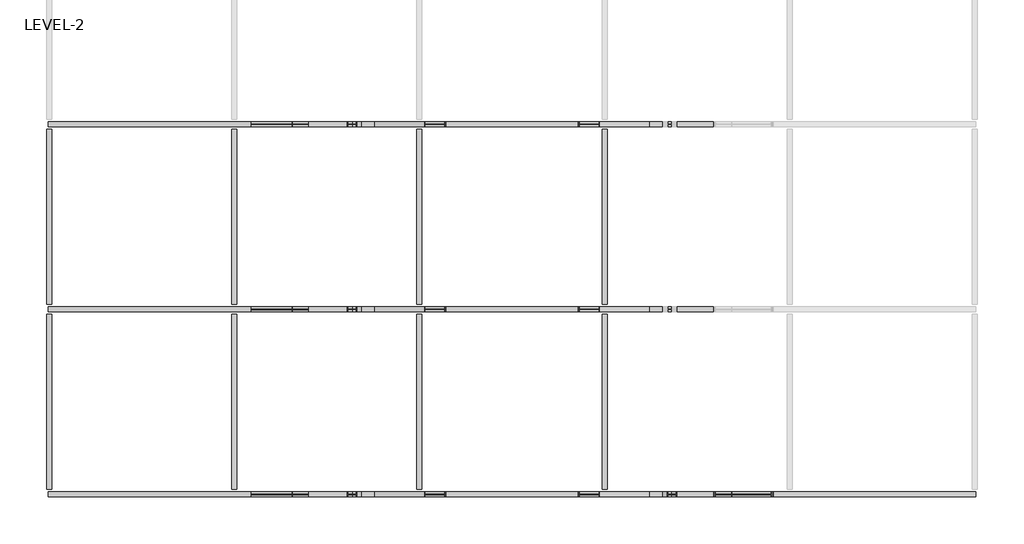
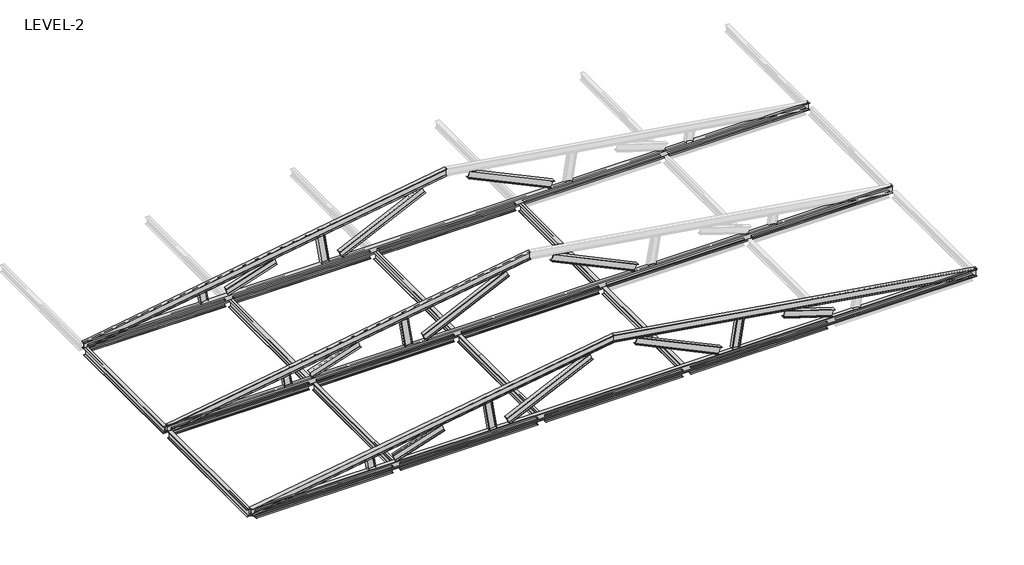
# One storey, part 1 of 3: 42 beams.
"""IFC4 building model written with IfcOpenShell, lengths in millimetres."""

from ifc_helpers import new_model, si_unit, frame, origin, place, context, project, spatial, polyline, circle_curve, ellipse_curve, transform, mapped, element, save
from ifc_brep_helpers import plane_surface, revolved_surface, advanced_brep
from components import ub_universal_beams_ub305x165x40_616d6e4e, ub_universal_beams_ub305x165x40_3f70edd5, ub_universal_beams_ub305x165x40_c9eec61f, ub_universal_beams_ub305x165x40_c956ba20, ub_universal_beams_ub305x165x40_f58164a9, ub_universal_beams_ub305x165x40_ef0a91e2, ub_universal_beams_ub305x165x40_83ed4f69, ub_universal_beams_ub305x165x40_46a3dc55, ub_universal_beams_ub305x165x40_0b6a72e4, ub_universal_beams_ub305x165x40_05d28e63

model = new_model("IFC4")

# Units and contexts
model_context = context("Model", 3, world=origin())
ifc_project = project(units=[si_unit("LENGTHUNIT", "METRE", prefix="MILLI")], contexts=[model_context])

# Site, building, storey
site = spatial("IfcSite", under=ifc_project)
building = spatial("IfcBuilding", under=site)
storey = spatial("IfcBuildingStorey", under=building, Name="LEVEL-2", Elevation=4267.0)

# Beams
placement = place(None, origin())
element("IfcBeam", 1, ObjectType="UB-Universal Beams : UB305x165x40", at=placement, inside=storey, context=model_context, shape_type="AdvancedBrep", body=[
    advanced_brep(
    [(-18518.3117021, -14245.9765895, 4127.2241081), (-18516.724958, -14245.9765895, 4117.1482834), (-18516.724958, -14410.9765895, 4117.1482834), (-18518.3117021, -14410.9765895, 4127.2241081), (-18518.3117021, -14340.3765895, 4127.2241081), (-18519.696214, -14331.4765895, 4136.0157591), (-18560.9515593, -14331.4765895, 4397.9872012), (-18562.3360712, -14340.3765895, 4406.7788522), (-18562.3360712, -14410.9765895, 4406.7788522), (-18563.9228153, -14410.9765895, 4416.8546768), (-18563.9228153, -14245.9765895, 4416.8546768), (-18562.3360712, -14245.9765895, 4406.7788522), (-18562.3360712, -14316.5765895, 4406.7788522), (-18560.9515593, -14325.4765895, 4397.9872012), (-18519.696214, -14325.4765895, 4136.0157591), (-18518.3117021, -14316.5765895, 4127.2241081), (-3300.3332854, -14316.5765895, 6523.7561422), (-3300.3332854, -14245.9765895, 6523.7561422), (-3300.3332854, -14325.4765895, 6532.7658266), (-3300.3332854, -14325.4765895, 6801.2341734), (-3300.3332854, -14316.5765895, 6810.2438578), (-3300.3332854, -14245.9765895, 6810.2438578), (-3300.3332854, -14245.9765895, 6820.5695634), (-3300.3332854, -14410.9765895, 6820.5695634), (-3300.3332854, -14410.9765895, 6810.2438578), (-3300.3332854, -14340.3765895, 6810.2438578), (-3300.3332854, -14331.4765895, 6801.2341734), (-3300.3332854, -14331.4765895, 6532.7658266), (-3300.3332854, -14340.3765895, 6523.7561422), (-3300.3332854, -14410.9765895, 6523.7561422), (-3300.3332854, -14410.9765895, 6513.4304366), (-3300.3332854, -14245.9765895, 6513.4304366)],
    [
        (0, 1),
        (1, 2),
        (2, 3),
        (3, 4),
        (4, 5, circle_curve(frame((-18519.696214, -14340.3765895, 4136.0157591), z_axis=(0.9878259507117182, 0.0, 0.1555631418443652), x_axis=(0.0, -1.0, 0.0)), 8.9)),
        (5, 6),
        (6, 7, circle_curve(frame((-18560.9515593, -14340.3765895, 4397.9872012), z_axis=(0.9878259507117182, 0.0, 0.1555631418443652), x_axis=(0.0, -1.0, 0.0)), 8.9)),
        (7, 8),
        (8, 9),
        (9, 10),
        (10, 11),
        (11, 12),
        (12, 13, circle_curve(frame((-18560.9515593, -14316.5765895, 4397.9872012), z_axis=(0.9878259507117182, 0.0, 0.1555631418443652), x_axis=(0.0, -1.0, 0.0)), 8.9)),
        (13, 14),
        (14, 15, circle_curve(frame((-18519.696214, -14316.5765895, 4136.0157591), z_axis=(0.9878259507117182, 0.0, 0.1555631418443652), x_axis=(0.0, -1.0, 0.0)), 8.9)),
        (15, 0),
        (16, 17),
        (17, 0),
        (15, 16),
        (18, 16, ellipse_curve(frame((-3300.3332854, -14316.5765895, 6532.7658266), z_axis=(1.0, 0.0, 0.0), x_axis=(0.0, 0.0, -1.0)), 9.0096843, 8.9)),
        (14, 18),
        (19, 18),
        (13, 19),
        (20, 19, ellipse_curve(frame((-3300.3332854, -14316.5765895, 6801.2341734), z_axis=(1.0, 0.0, 0.0), x_axis=(0.0, 0.0, -1.0)), 9.0096843, 8.9)),
        (12, 20),
        (21, 20),
        (11, 21),
        (22, 21),
        (10, 22),
        (23, 22),
        (9, 23),
        (24, 23),
        (8, 24),
        (25, 24),
        (7, 25),
        (26, 25, ellipse_curve(frame((-3300.3332854, -14340.3765895, 6801.2341734), z_axis=(1.0, 0.0, 0.0), x_axis=(0.0, 0.0, -1.0)), 9.0096843, 8.9)),
        (6, 26),
        (27, 26),
        (5, 27),
        (28, 27, ellipse_curve(frame((-3300.3332854, -14340.3765895, 6532.7658266), z_axis=(1.0, 0.0, 0.0), x_axis=(0.0, 0.0, -1.0)), 9.0096843, 8.9)),
        (4, 28),
        (29, 28),
        (3, 29),
        (30, 29),
        (2, 30),
        (31, 30),
        (1, 31),
        (17, 31),
    ],
    [
        plane_surface(frame((-18540.3238866, -14328.4765895, 4267.0014801), z_axis=(-0.9878259507117182, 0.0, -0.1555631418443652), x_axis=(-0.1555631418443652, 0.0, 0.9878259507117182))),
        plane_surface(frame((-3278.3304997, -14245.9765895, 6527.2211478), z_axis=(-0.1555631418443652, 0.0, 0.9878259507117182), x_axis=(-0.9878259507117182, 0.0, -0.1555631418443652))),
        revolved_surface(polyline([(-18519.696214059466, -14325.4765895, 4136.015759042602), (-3298.948773435937, -14325.4765895, 6532.983859928199)]), (-3279.7150116, -14316.5765895, 6536.0127988), (-0.9878259507117182, 0.0, -0.1555631418443652)),
        plane_surface(frame((-3279.7150116, -14325.4765895, 6536.0127988), z_axis=(0.0, 1.0, 0.0), x_axis=(-0.9878259507117182, 0.0, -0.1555631418443652))),
        revolved_surface(polyline([(-18560.95155929262, -14325.4765895, 4397.98720115313), (-3298.948773431581, -14325.4765895, 6801.452206800539)]), (-3320.9703569, -14316.5765895, 6797.9842409), (-0.9878259507117182, 0.0, -0.1555631418443652)),
        plane_surface(frame((-3322.3548688, -14316.5765895, 6806.7758919), z_axis=(0.1555631418443652, 0.0, -0.9878259507117182), x_axis=(-0.9878259507117182, 0.0, -0.1555631418443652))),
        plane_surface(frame((-3322.3548688, -14245.9765895, 6806.7758919), z_axis=(0.0, 1.0, 0.0), x_axis=(-0.9878259507117182, 0.0, -0.1555631418443652))),
        plane_surface(frame((-3323.9416129, -14245.9765895, 6816.8517166), z_axis=(-0.1555631418443652, 0.0, 0.9878259507117182), x_axis=(-0.9878259507117182, 0.0, -0.1555631418443652))),
        plane_surface(frame((-3323.9416129, -14410.9765895, 6816.8517166), z_axis=(0.0, -1.0, 0.0), x_axis=(-0.9878259507117182, 0.0, -0.1555631418443652))),
        plane_surface(frame((-3322.3548688, -14410.9765895, 6806.7758919), z_axis=(0.1555631418443652, 0.0, -0.9878259507117182), x_axis=(-0.9878259507117182, 0.0, -0.1555631418443652))),
        revolved_surface(polyline([(-18560.95155929262, -14349.2765895, 4397.98720115313), (-3298.948773431581, -14349.2765895, 6801.452206800539)]), (-3320.9703569, -14340.3765895, 6797.9842409), (-0.9878259507117182, 0.0, -0.1555631418443652)),
        plane_surface(frame((-3320.9703569, -14331.4765895, 6797.9842409), z_axis=(0.0, -1.0, 0.0), x_axis=(-0.9878259507117182, 0.0, -0.1555631418443652))),
        revolved_surface(polyline([(-18519.696214059466, -14349.2765895, 4136.015759042602), (-3298.948773435937, -14349.2765895, 6532.983859928199)]), (-3279.7150116, -14340.3765895, 6536.0127988), (-0.9878259507117182, 0.0, -0.1555631418443652)),
        plane_surface(frame((-3278.3304997, -14340.3765895, 6527.2211478), z_axis=(-0.1555631418443652, 0.0, 0.9878259507117182), x_axis=(-0.9878259507117182, 0.0, -0.1555631418443652))),
        plane_surface(frame((-3278.3304997, -14410.9765895, 6527.2211478), z_axis=(0.0, -1.0, 0.0), x_axis=(-0.9878259507117182, 0.0, -0.1555631418443652))),
        plane_surface(frame((-3276.7437556, -14410.9765895, 6517.1453232), z_axis=(0.1555631418443652, 0.0, -0.9878259507117182), x_axis=(-0.9878259507117182, 0.0, -0.1555631418443652))),
        plane_surface(frame((-3276.7437556, -14245.9765895, 6517.1453232), z_axis=(0.0, 1.0, 0.0), x_axis=(-0.9878259507117182, 0.0, -0.1555631418443652))),
        plane_surface(frame((-3300.3332854, -14328.4765895, 6820.5695634), z_axis=(1.0, 0.0, 0.0), x_axis=(0.0, -1.0, 0.0))),
    ],
    [
        (0, [[1, 2, 3, 4, 5, 6, 7, 8, 9, 10, 11, 12, 13, 14, 15, 16]]),
        (1, [[17, 18, -16, 19]]),
        (2, [[20, -19, -15, 21]]),
        (3, [[22, -21, -14, 23]]),
        (4, [[24, -23, -13, 25]]),
        (5, [[26, -25, -12, 27]]),
        (6, [[28, -27, -11, 29]]),
        (7, [[30, -29, -10, 31]]),
        (8, [[32, -31, -9, 33]]),
        (9, [[34, -33, -8, 35]]),
        (10, [[36, -35, -7, 37]]),
        (11, [[38, -37, -6, 39]]),
        (12, [[40, -39, -5, 41]]),
        (13, [[42, -41, -4, 43]]),
        (14, [[44, -43, -3, 45]]),
        (15, [[46, -45, -2, 47]]),
        (16, [[48, -47, -1, -18]]),
        (17, [[-17, -20, -22, -24, -26, -28, -30, -32, -34, -36, -38, -40, -42, -44, -46, -48]]),
    ],
),
])
element("IfcBeam", 2, ObjectType="UB-Universal Beams : UB305x165x40", at=placement, inside=storey, context=model_context, shape_type="AdvancedBrep", body=[
    advanced_brep(
    [(11917.6451312, -14245.9765895, 4127.2241081), (11917.6451312, -14316.5765895, 4127.2241081), (11919.0296431, -14325.4765895, 4136.0157591), (11960.2849884, -14325.4765895, 4397.9872012), (11961.6695003, -14316.5765895, 4406.7788522), (11961.6695003, -14245.9765895, 4406.7788522), (11963.2562444, -14245.9765895, 4416.8546768), (11963.2562444, -14410.9765895, 4416.8546768), (11961.6695003, -14410.9765895, 4406.7788522), (11961.6695003, -14340.3765895, 4406.7788522), (11960.2849884, -14331.4765895, 4397.9872012), (11919.0296431, -14331.4765895, 4136.0157591), (11917.6451312, -14340.3765895, 4127.2241081), (11917.6451312, -14410.9765895, 4127.2241081), (11916.0583871, -14410.9765895, 4117.1482834), (11916.0583871, -14245.9765895, 4117.1482834), (-3300.3332854, -14245.9765895, 6523.7561422), (-3300.3332854, -14316.5765895, 6523.7561422), (-3300.3332854, -14325.4765895, 6532.7658266), (-3300.3332854, -14325.4765895, 6801.2341734), (-3300.3332854, -14316.5765895, 6810.2438578), (-3300.3332854, -14245.9765895, 6810.2438578), (-3300.3332854, -14245.9765895, 6820.5695634), (-3300.3332854, -14410.9765895, 6820.5695634), (-3300.3332854, -14410.9765895, 6810.2438578), (-3300.3332854, -14340.3765895, 6810.2438578), (-3300.3332854, -14331.4765895, 6801.2341734), (-3300.3332854, -14331.4765895, 6532.7658266), (-3300.3332854, -14340.3765895, 6523.7561422), (-3300.3332854, -14410.9765895, 6523.7561422), (-3300.3332854, -14410.9765895, 6513.4304366), (-3300.3332854, -14245.9765895, 6513.4304366)],
    [
        (0, 1),
        (1, 2, circle_curve(frame((11919.0296431, -14316.5765895, 4136.0157591), z_axis=(-0.9878259507117182, 0.0, 0.1555631418443652), x_axis=(0.0, -1.0, 0.0)), 8.9)),
        (2, 3),
        (3, 4, circle_curve(frame((11960.2849884, -14316.5765895, 4397.9872012), z_axis=(-0.9878259507117182, 0.0, 0.1555631418443652), x_axis=(0.0, -1.0, 0.0)), 8.9)),
        (4, 5),
        (5, 6),
        (6, 7),
        (7, 8),
        (8, 9),
        (9, 10, circle_curve(frame((11960.2849884, -14340.3765895, 4397.9872012), z_axis=(-0.9878259507117182, 0.0, 0.1555631418443652), x_axis=(0.0, -1.0, 0.0)), 8.9)),
        (10, 11),
        (11, 12, circle_curve(frame((11919.0296431, -14340.3765895, 4136.0157591), z_axis=(-0.9878259507117182, 0.0, 0.1555631418443652), x_axis=(0.0, -1.0, 0.0)), 8.9)),
        (12, 13),
        (13, 14),
        (14, 15),
        (15, 0),
        (0, 16),
        (16, 17),
        (17, 1),
        (17, 18, ellipse_curve(frame((-3300.3332854, -14316.5765895, 6532.7658266), z_axis=(-1.0, 0.0, 0.0), x_axis=(0.0, 0.0, 1.0)), 9.0096843, 8.9)),
        (18, 2),
        (18, 19),
        (19, 3),
        (19, 20, ellipse_curve(frame((-3300.3332854, -14316.5765895, 6801.2341734), z_axis=(-1.0, 0.0, 0.0), x_axis=(0.0, 0.0, 1.0)), 9.0096843, 8.9)),
        (20, 4),
        (20, 21),
        (21, 5),
        (21, 22),
        (22, 6),
        (22, 23),
        (23, 7),
        (23, 24),
        (24, 8),
        (24, 25),
        (25, 9),
        (25, 26, ellipse_curve(frame((-3300.3332854, -14340.3765895, 6801.2341734), z_axis=(-1.0, 0.0, 0.0), x_axis=(0.0, 0.0, 1.0)), 9.0096843, 8.9)),
        (26, 10),
        (26, 27),
        (27, 11),
        (27, 28, ellipse_curve(frame((-3300.3332854, -14340.3765895, 6532.7658266), z_axis=(-1.0, 0.0, 0.0), x_axis=(0.0, 0.0, 1.0)), 9.0096843, 8.9)),
        (28, 12),
        (28, 29),
        (29, 13),
        (29, 30),
        (30, 14),
        (30, 31),
        (31, 15),
        (31, 16),
    ],
    [
        plane_surface(frame((11939.6573157, -14328.4765895, 4267.0014801), z_axis=(0.9878259507117182, 0.0, -0.1555631418443652), x_axis=(0.1555631418443652, 0.0, 0.9878259507117182))),
        plane_surface(frame((11917.6451312, -14245.9765895, 4127.2241081), z_axis=(0.1555631418443652, 0.0, 0.9878259507117182), x_axis=(-0.9878259507117182, 0.0, 0.1555631418443652))),
        revolved_surface(polyline([(-3301.7177973591024, -14325.4765895, 6532.983859959702), (11919.029643166847, -14325.4765895, 4136.015759089472)]), (11919.0296431, -14316.5765895, 4136.0157591), (-0.9878259507117182, 0.0, 0.1555631418443652)),
        plane_surface(frame((11919.0296431, -14325.4765895, 4136.0157591), z_axis=(0.0, 1.0, 0.0), x_axis=(-0.9878259507117182, 0.0, 0.1555631418443652))),
        revolved_surface(polyline([(-3301.717797363457, -14325.4765895, 6801.452206832042), (11960.2849884, -14325.4765895, 4397.9872012)]), (11960.2849884, -14316.5765895, 4397.9872012), (-0.9878259507117182, 0.0, 0.1555631418443652)),
        plane_surface(frame((11961.6695003, -14316.5765895, 4406.7788522), z_axis=(-0.1555631418443652, 0.0, -0.9878259507117182), x_axis=(-0.9878259507117182, 0.0, 0.1555631418443652))),
        plane_surface(frame((11961.6695003, -14245.9765895, 4406.7788522), z_axis=(0.0, 1.0, 0.0), x_axis=(-0.9878259507117182, 0.0, 0.1555631418443652))),
        plane_surface(frame((11963.2562444, -14245.9765895, 4416.8546768), z_axis=(0.1555631418443652, 0.0, 0.9878259507117182), x_axis=(-0.9878259507117182, 0.0, 0.1555631418443652))),
        plane_surface(frame((11963.2562444, -14410.9765895, 4416.8546768), z_axis=(0.0, -1.0, 0.0), x_axis=(-0.9878259507117182, 0.0, 0.1555631418443652))),
        plane_surface(frame((11961.6695003, -14410.9765895, 4406.7788522), z_axis=(-0.1555631418443652, 0.0, -0.9878259507117182), x_axis=(-0.9878259507117182, 0.0, 0.1555631418443652))),
        revolved_surface(polyline([(-3301.717797363457, -14349.2765895, 6801.452206832042), (11960.2849884, -14349.2765895, 4397.9872012)]), (11960.2849884, -14340.3765895, 4397.9872012), (-0.9878259507117182, 0.0, 0.1555631418443652)),
        plane_surface(frame((11960.2849884, -14331.4765895, 4397.9872012), z_axis=(0.0, -1.0, 0.0), x_axis=(-0.9878259507117182, 0.0, 0.1555631418443652))),
        revolved_surface(polyline([(-3301.7177973591024, -14349.2765895, 6532.983859959702), (11919.029643166847, -14349.2765895, 4136.015759089472)]), (11919.0296431, -14340.3765895, 4136.0157591), (-0.9878259507117182, 0.0, 0.1555631418443652)),
        plane_surface(frame((11917.6451312, -14340.3765895, 4127.2241081), z_axis=(0.1555631418443652, 0.0, 0.9878259507117182), x_axis=(-0.9878259507117182, 0.0, 0.1555631418443652))),
        plane_surface(frame((11917.6451312, -14410.9765895, 4127.2241081), z_axis=(0.0, -1.0, 0.0), x_axis=(-0.9878259507117182, 0.0, 0.1555631418443652))),
        plane_surface(frame((11916.0583871, -14410.9765895, 4117.1482834), z_axis=(-0.1555631418443652, 0.0, -0.9878259507117182), x_axis=(-0.9878259507117182, 0.0, 0.1555631418443652))),
        plane_surface(frame((11916.0583871, -14245.9765895, 4117.1482834), z_axis=(0.0, 1.0, 0.0), x_axis=(-0.9878259507117182, 0.0, 0.1555631418443652))),
        plane_surface(frame((-3300.3332854, -14328.4765895, 6820.5695634), z_axis=(-1.0, 0.0, 0.0), x_axis=(0.0, 1.0, 0.0))),
    ],
    [
        (0, [[1, 2, 3, 4, 5, 6, 7, 8, 9, 10, 11, 12, 13, 14, 15, 16]]),
        (1, [[-1, 17, 18, 19]]),
        (2, [[-2, -19, 20, 21]]),
        (3, [[-3, -21, 22, 23]]),
        (4, [[-4, -23, 24, 25]]),
        (5, [[-5, -25, 26, 27]]),
        (6, [[-6, -27, 28, 29]]),
        (7, [[-7, -29, 30, 31]]),
        (8, [[-8, -31, 32, 33]]),
        (9, [[-9, -33, 34, 35]]),
        (10, [[-10, -35, 36, 37]]),
        (11, [[-11, -37, 38, 39]]),
        (12, [[-12, -39, 40, 41]]),
        (13, [[-13, -41, 42, 43]]),
        (14, [[-14, -43, 44, 45]]),
        (15, [[-15, -45, 46, 47]]),
        (16, [[-16, -47, 48, -17]]),
        (17, [[-48, -46, -44, -42, -40, -38, -36, -34, -32, -30, -28, -26, -24, -22, -20, -18]]),
    ],
),
])
element("IfcBeam", 3, ObjectType="UB-Universal Beams : UB305x165x40", at=placement, inside=storey, context=model_context, shape_type="AdvancedBrep", body=[
    advanced_brep(
    [(-18518.3117021, -8149.9765895, 4127.2241081), (-18516.724958, -8149.9765895, 4117.1482834), (-18516.724958, -8314.9765895, 4117.1482834), (-18518.3117021, -8314.9765895, 4127.2241081), (-18518.3117021, -8244.3765895, 4127.2241081), (-18519.696214, -8235.4765895, 4136.0157591), (-18560.9515593, -8235.4765895, 4397.9872012), (-18562.3360712, -8244.3765895, 4406.7788522), (-18562.3360712, -8314.9765895, 4406.7788522), (-18563.9228153, -8314.9765895, 4416.8546768), (-18563.9228153, -8149.9765895, 4416.8546768), (-18562.3360712, -8149.9765895, 4406.7788522), (-18562.3360712, -8220.5765895, 4406.7788522), (-18560.9515593, -8229.4765895, 4397.9872012), (-18519.696214, -8229.4765895, 4136.0157591), (-18518.3117021, -8220.5765895, 4127.2241081), (-3300.3332854, -8220.5765895, 6523.7561422), (-3300.3332854, -8149.9765895, 6523.7561422), (-3300.3332854, -8229.4765895, 6532.7658266), (-3300.3332854, -8229.4765895, 6801.2341734), (-3300.3332854, -8220.5765895, 6810.2438578), (-3300.3332854, -8149.9765895, 6810.2438578), (-3300.3332854, -8149.9765895, 6820.5695634), (-3300.3332854, -8314.9765895, 6820.5695634), (-3300.3332854, -8314.9765895, 6810.2438578), (-3300.3332854, -8244.3765895, 6810.2438578), (-3300.3332854, -8235.4765895, 6801.2341734), (-3300.3332854, -8235.4765895, 6532.7658266), (-3300.3332854, -8244.3765895, 6523.7561422), (-3300.3332854, -8314.9765895, 6523.7561422), (-3300.3332854, -8314.9765895, 6513.4304366), (-3300.3332854, -8149.9765895, 6513.4304366)],
    [
        (0, 1),
        (1, 2),
        (2, 3),
        (3, 4),
        (4, 5, circle_curve(frame((-18519.696214, -8244.3765895, 4136.0157591), z_axis=(0.9878259507117182, 0.0, 0.1555631418443652), x_axis=(0.0, -1.0, 0.0)), 8.9)),
        (5, 6),
        (6, 7, circle_curve(frame((-18560.9515593, -8244.3765895, 4397.9872012), z_axis=(0.9878259507117182, 0.0, 0.1555631418443652), x_axis=(0.0, -1.0, 0.0)), 8.9)),
        (7, 8),
        (8, 9),
        (9, 10),
        (10, 11),
        (11, 12),
        (12, 13, circle_curve(frame((-18560.9515593, -8220.5765895, 4397.9872012), z_axis=(0.9878259507117182, 0.0, 0.1555631418443652), x_axis=(0.0, -1.0, 0.0)), 8.9)),
        (13, 14),
        (14, 15, circle_curve(frame((-18519.696214, -8220.5765895, 4136.0157591), z_axis=(0.9878259507117182, 0.0, 0.1555631418443652), x_axis=(0.0, -1.0, 0.0)), 8.9)),
        (15, 0),
        (16, 17),
        (17, 0),
        (15, 16),
        (18, 16, ellipse_curve(frame((-3300.3332854, -8220.5765895, 6532.7658266), z_axis=(1.0, 0.0, 0.0), x_axis=(0.0, 0.0, -1.0)), 9.0096843, 8.9)),
        (14, 18),
        (19, 18),
        (13, 19),
        (20, 19, ellipse_curve(frame((-3300.3332854, -8220.5765895, 6801.2341734), z_axis=(1.0, 0.0, 0.0), x_axis=(0.0, 0.0, -1.0)), 9.0096843, 8.9)),
        (12, 20),
        (21, 20),
        (11, 21),
        (22, 21),
        (10, 22),
        (23, 22),
        (9, 23),
        (24, 23),
        (8, 24),
        (25, 24),
        (7, 25),
        (26, 25, ellipse_curve(frame((-3300.3332854, -8244.3765895, 6801.2341734), z_axis=(1.0, 0.0, 0.0), x_axis=(0.0, 0.0, -1.0)), 9.0096843, 8.9)),
        (6, 26),
        (27, 26),
        (5, 27),
        (28, 27, ellipse_curve(frame((-3300.3332854, -8244.3765895, 6532.7658266), z_axis=(1.0, 0.0, 0.0), x_axis=(0.0, 0.0, -1.0)), 9.0096843, 8.9)),
        (4, 28),
        (29, 28),
        (3, 29),
        (30, 29),
        (2, 30),
        (31, 30),
        (1, 31),
        (17, 31),
    ],
    [
        plane_surface(frame((-18540.3238866, -8232.4765895, 4267.0014801), z_axis=(-0.9878259507117182, 0.0, -0.1555631418443652), x_axis=(-0.1555631418443652, 0.0, 0.9878259507117182))),
        plane_surface(frame((-3278.3304997, -8149.9765895, 6527.2211478), z_axis=(-0.1555631418443652, 0.0, 0.9878259507117182), x_axis=(-0.9878259507117182, 0.0, -0.1555631418443652))),
        revolved_surface(polyline([(-18519.696214059466, -8229.4765895, 4136.015759042602), (-3298.948773435937, -8229.4765895, 6532.983859928199)]), (-3279.7150116, -8220.5765895, 6536.0127988), (-0.9878259507117182, 0.0, -0.1555631418443652)),
        plane_surface(frame((-3279.7150116, -8229.4765895, 6536.0127988), z_axis=(0.0, 1.0, 0.0), x_axis=(-0.9878259507117182, 0.0, -0.1555631418443652))),
        revolved_surface(polyline([(-18560.95155929262, -8229.4765895, 4397.98720115313), (-3298.948773431581, -8229.4765895, 6801.452206800539)]), (-3320.9703569, -8220.5765895, 6797.9842409), (-0.9878259507117182, 0.0, -0.1555631418443652)),
        plane_surface(frame((-3322.3548688, -8220.5765895, 6806.7758919), z_axis=(0.1555631418443652, 0.0, -0.9878259507117182), x_axis=(-0.9878259507117182, 0.0, -0.1555631418443652))),
        plane_surface(frame((-3322.3548688, -8149.9765895, 6806.7758919), z_axis=(0.0, 1.0, 0.0), x_axis=(-0.9878259507117182, 0.0, -0.1555631418443652))),
        plane_surface(frame((-3323.9416129, -8149.9765895, 6816.8517166), z_axis=(-0.1555631418443652, 0.0, 0.9878259507117182), x_axis=(-0.9878259507117182, 0.0, -0.1555631418443652))),
        plane_surface(frame((-3323.9416129, -8314.9765895, 6816.8517166), z_axis=(0.0, -1.0, 0.0), x_axis=(-0.9878259507117182, 0.0, -0.1555631418443652))),
        plane_surface(frame((-3322.3548688, -8314.9765895, 6806.7758919), z_axis=(0.1555631418443652, 0.0, -0.9878259507117182), x_axis=(-0.9878259507117182, 0.0, -0.1555631418443652))),
        revolved_surface(polyline([(-18560.95155929262, -8253.2765895, 4397.98720115313), (-3298.948773431581, -8253.2765895, 6801.452206800539)]), (-3320.9703569, -8244.3765895, 6797.9842409), (-0.9878259507117182, 0.0, -0.1555631418443652)),
        plane_surface(frame((-3320.9703569, -8235.4765895, 6797.9842409), z_axis=(0.0, -1.0, 0.0), x_axis=(-0.9878259507117182, 0.0, -0.1555631418443652))),
        revolved_surface(polyline([(-18519.696214059466, -8253.2765895, 4136.015759042602), (-3298.948773435937, -8253.2765895, 6532.983859928199)]), (-3279.7150116, -8244.3765895, 6536.0127988), (-0.9878259507117182, 0.0, -0.1555631418443652)),
        plane_surface(frame((-3278.3304997, -8244.3765895, 6527.2211478), z_axis=(-0.1555631418443652, 0.0, 0.9878259507117182), x_axis=(-0.9878259507117182, 0.0, -0.1555631418443652))),
        plane_surface(frame((-3278.3304997, -8314.9765895, 6527.2211478), z_axis=(0.0, -1.0, 0.0), x_axis=(-0.9878259507117182, 0.0, -0.1555631418443652))),
        plane_surface(frame((-3276.7437556, -8314.9765895, 6517.1453232), z_axis=(0.1555631418443652, 0.0, -0.9878259507117182), x_axis=(-0.9878259507117182, 0.0, -0.1555631418443652))),
        plane_surface(frame((-3276.7437556, -8149.9765895, 6517.1453232), z_axis=(0.0, 1.0, 0.0), x_axis=(-0.9878259507117182, 0.0, -0.1555631418443652))),
        plane_surface(frame((-3300.3332854, -8232.4765895, 6820.5695634), z_axis=(1.0, 0.0, 0.0), x_axis=(0.0, -1.0, 0.0))),
    ],
    [
        (0, [[1, 2, 3, 4, 5, 6, 7, 8, 9, 10, 11, 12, 13, 14, 15, 16]]),
        (1, [[17, 18, -16, 19]]),
        (2, [[20, -19, -15, 21]]),
        (3, [[22, -21, -14, 23]]),
        (4, [[24, -23, -13, 25]]),
        (5, [[26, -25, -12, 27]]),
        (6, [[28, -27, -11, 29]]),
        (7, [[30, -29, -10, 31]]),
        (8, [[32, -31, -9, 33]]),
        (9, [[34, -33, -8, 35]]),
        (10, [[36, -35, -7, 37]]),
        (11, [[38, -37, -6, 39]]),
        (12, [[40, -39, -5, 41]]),
        (13, [[42, -41, -4, 43]]),
        (14, [[44, -43, -3, 45]]),
        (15, [[46, -45, -2, 47]]),
        (16, [[48, -47, -1, -18]]),
        (17, [[-17, -20, -22, -24, -26, -28, -30, -32, -34, -36, -38, -40, -42, -44, -46, -48]]),
    ],
),
])
element("IfcBeam", 4, ObjectType="UB-Universal Beams : UB305x165x40", at=placement, inside=storey, context=model_context, shape_type="AdvancedBrep", body=[
    advanced_brep(
    [(-18518.3117021, -2053.9765895, 4127.2241081), (-18516.724958, -2053.9765895, 4117.1482834), (-18516.724958, -2218.9765895, 4117.1482834), (-18518.3117021, -2218.9765895, 4127.2241081), (-18518.3117021, -2148.3765895, 4127.2241081), (-18519.696214, -2139.4765895, 4136.0157591), (-18560.9515593, -2139.4765895, 4397.9872012), (-18562.3360712, -2148.3765895, 4406.7788522), (-18562.3360712, -2218.9765895, 4406.7788522), (-18563.9228153, -2218.9765895, 4416.8546768), (-18563.9228153, -2053.9765895, 4416.8546768), (-18562.3360712, -2053.9765895, 4406.7788522), (-18562.3360712, -2124.5765895, 4406.7788522), (-18560.9515593, -2133.4765895, 4397.9872012), (-18519.696214, -2133.4765895, 4136.0157591), (-18518.3117021, -2124.5765895, 4127.2241081), (-3300.3332854, -2124.5765895, 6523.7561422), (-3300.3332854, -2053.9765895, 6523.7561422), (-3300.3332854, -2133.4765895, 6532.7658266), (-3300.3332854, -2133.4765895, 6801.2341734), (-3300.3332854, -2124.5765895, 6810.2438578), (-3300.3332854, -2053.9765895, 6810.2438578), (-3300.3332854, -2053.9765895, 6820.5695634), (-3300.3332854, -2218.9765895, 6820.5695634), (-3300.3332854, -2218.9765895, 6810.2438578), (-3300.3332854, -2148.3765895, 6810.2438578), (-3300.3332854, -2139.4765895, 6801.2341734), (-3300.3332854, -2139.4765895, 6532.7658266), (-3300.3332854, -2148.3765895, 6523.7561422), (-3300.3332854, -2218.9765895, 6523.7561422), (-3300.3332854, -2218.9765895, 6513.4304366), (-3300.3332854, -2053.9765895, 6513.4304366)],
    [
        (0, 1),
        (1, 2),
        (2, 3),
        (3, 4),
        (4, 5, circle_curve(frame((-18519.696214, -2148.3765895, 4136.0157591), z_axis=(0.9878259507117182, 0.0, 0.1555631418443652), x_axis=(0.0, -1.0, 0.0)), 8.9)),
        (5, 6),
        (6, 7, circle_curve(frame((-18560.9515593, -2148.3765895, 4397.9872012), z_axis=(0.9878259507117182, 0.0, 0.1555631418443652), x_axis=(0.0, -1.0, 0.0)), 8.9)),
        (7, 8),
        (8, 9),
        (9, 10),
        (10, 11),
        (11, 12),
        (12, 13, circle_curve(frame((-18560.9515593, -2124.5765895, 4397.9872012), z_axis=(0.9878259507117182, 0.0, 0.1555631418443652), x_axis=(0.0, -1.0, 0.0)), 8.9)),
        (13, 14),
        (14, 15, circle_curve(frame((-18519.696214, -2124.5765895, 4136.0157591), z_axis=(0.9878259507117182, 0.0, 0.1555631418443652), x_axis=(0.0, -1.0, 0.0)), 8.9)),
        (15, 0),
        (16, 17),
        (17, 0),
        (15, 16),
        (18, 16, ellipse_curve(frame((-3300.3332854, -2124.5765895, 6532.7658266), z_axis=(1.0, 0.0, 0.0), x_axis=(0.0, 0.0, -1.0)), 9.0096843, 8.9)),
        (14, 18),
        (19, 18),
        (13, 19),
        (20, 19, ellipse_curve(frame((-3300.3332854, -2124.5765895, 6801.2341734), z_axis=(1.0, 0.0, 0.0), x_axis=(0.0, 0.0, -1.0)), 9.0096843, 8.9)),
        (12, 20),
        (21, 20),
        (11, 21),
        (22, 21),
        (10, 22),
        (23, 22),
        (9, 23),
        (24, 23),
        (8, 24),
        (25, 24),
        (7, 25),
        (26, 25, ellipse_curve(frame((-3300.3332854, -2148.3765895, 6801.2341734), z_axis=(1.0, 0.0, 0.0), x_axis=(0.0, 0.0, -1.0)), 9.0096843, 8.9)),
        (6, 26),
        (27, 26),
        (5, 27),
        (28, 27, ellipse_curve(frame((-3300.3332854, -2148.3765895, 6532.7658266), z_axis=(1.0, 0.0, 0.0), x_axis=(0.0, 0.0, -1.0)), 9.0096843, 8.9)),
        (4, 28),
        (29, 28),
        (3, 29),
        (30, 29),
        (2, 30),
        (31, 30),
        (1, 31),
        (17, 31),
    ],
    [
        plane_surface(frame((-18540.3238866, -2136.4765895, 4267.0014801), z_axis=(-0.9878259507117182, 0.0, -0.1555631418443652), x_axis=(-0.1555631418443652, 0.0, 0.9878259507117182))),
        plane_surface(frame((-3278.3304997, -2053.9765895, 6527.2211478), z_axis=(-0.1555631418443652, 0.0, 0.9878259507117182), x_axis=(-0.9878259507117182, 0.0, -0.1555631418443652))),
        revolved_surface(polyline([(-18519.696214059466, -2133.4765895, 4136.015759042602), (-3298.948773435937, -2133.4765895, 6532.983859928199)]), (-3279.7150116, -2124.5765895, 6536.0127988), (-0.9878259507117182, 0.0, -0.1555631418443652)),
        plane_surface(frame((-3279.7150116, -2133.4765895, 6536.0127988), z_axis=(0.0, 1.0, 0.0), x_axis=(-0.9878259507117182, 0.0, -0.1555631418443652))),
        revolved_surface(polyline([(-18560.95155929262, -2133.4765895, 4397.98720115313), (-3298.948773431581, -2133.4765895, 6801.452206800539)]), (-3320.9703569, -2124.5765895, 6797.9842409), (-0.9878259507117182, 0.0, -0.1555631418443652)),
        plane_surface(frame((-3322.3548688, -2124.5765895, 6806.7758919), z_axis=(0.1555631418443652, 0.0, -0.9878259507117182), x_axis=(-0.9878259507117182, 0.0, -0.1555631418443652))),
        plane_surface(frame((-3322.3548688, -2053.9765895, 6806.7758919), z_axis=(0.0, 1.0, 0.0), x_axis=(-0.9878259507117182, 0.0, -0.1555631418443652))),
        plane_surface(frame((-3323.9416129, -2053.9765895, 6816.8517166), z_axis=(-0.1555631418443652, 0.0, 0.9878259507117182), x_axis=(-0.9878259507117182, 0.0, -0.1555631418443652))),
        plane_surface(frame((-3323.9416129, -2218.9765895, 6816.8517166), z_axis=(0.0, -1.0, 0.0), x_axis=(-0.9878259507117182, 0.0, -0.1555631418443652))),
        plane_surface(frame((-3322.3548688, -2218.9765895, 6806.7758919), z_axis=(0.1555631418443652, 0.0, -0.9878259507117182), x_axis=(-0.9878259507117182, 0.0, -0.1555631418443652))),
        revolved_surface(polyline([(-18560.95155929262, -2157.2765895000002, 4397.98720115313), (-3298.948773431581, -2157.2765895000002, 6801.452206800539)]), (-3320.9703569, -2148.3765895, 6797.9842409), (-0.9878259507117182, 0.0, -0.1555631418443652)),
        plane_surface(frame((-3320.9703569, -2139.4765895, 6797.9842409), z_axis=(0.0, -1.0, 0.0), x_axis=(-0.9878259507117182, 0.0, -0.1555631418443652))),
        revolved_surface(polyline([(-18519.696214059466, -2157.2765895000002, 4136.015759042602), (-3298.948773435937, -2157.2765895000002, 6532.983859928199)]), (-3279.7150116, -2148.3765895, 6536.0127988), (-0.9878259507117182, 0.0, -0.1555631418443652)),
        plane_surface(frame((-3278.3304997, -2148.3765895, 6527.2211478), z_axis=(-0.1555631418443652, 0.0, 0.9878259507117182), x_axis=(-0.9878259507117182, 0.0, -0.1555631418443652))),
        plane_surface(frame((-3278.3304997, -2218.9765895, 6527.2211478), z_axis=(0.0, -1.0, 0.0), x_axis=(-0.9878259507117182, 0.0, -0.1555631418443652))),
        plane_surface(frame((-3276.7437556, -2218.9765895, 6517.1453232), z_axis=(0.1555631418443652, 0.0, -0.9878259507117182), x_axis=(-0.9878259507117182, 0.0, -0.1555631418443652))),
        plane_surface(frame((-3276.7437556, -2053.9765895, 6517.1453232), z_axis=(0.0, 1.0, 0.0), x_axis=(-0.9878259507117182, 0.0, -0.1555631418443652))),
        plane_surface(frame((-3300.3332854, -2136.4765895, 6820.5695634), z_axis=(1.0, 0.0, 0.0), x_axis=(0.0, -1.0, 0.0))),
    ],
    [
        (0, [[1, 2, 3, 4, 5, 6, 7, 8, 9, 10, 11, 12, 13, 14, 15, 16]]),
        (1, [[17, 18, -16, 19]]),
        (2, [[20, -19, -15, 21]]),
        (3, [[22, -21, -14, 23]]),
        (4, [[24, -23, -13, 25]]),
        (5, [[26, -25, -12, 27]]),
        (6, [[28, -27, -11, 29]]),
        (7, [[30, -29, -10, 31]]),
        (8, [[32, -31, -9, 33]]),
        (9, [[34, -33, -8, 35]]),
        (10, [[36, -35, -7, 37]]),
        (11, [[38, -37, -6, 39]]),
        (12, [[40, -39, -5, 41]]),
        (13, [[42, -41, -4, 43]]),
        (14, [[44, -43, -3, 45]]),
        (15, [[46, -45, -2, 47]]),
        (16, [[48, -47, -1, -18]]),
        (17, [[-17, -20, -22, -24, -26, -28, -30, -32, -34, -36, -38, -40, -42, -44, -46, -48]]),
    ],
),
])
ub_universal_beams_ub305x165x40_shape = ub_universal_beams_ub305x165x40_616d6e4e(model_context)
element("IfcBeam", 5, ObjectType="UB-Universal Beams : UB305x165x40", at=placement, inside=storey, context=model_context, shape_type="MappedRepresentation", body=[
    mapped(ub_universal_beams_ub305x165x40_shape, transform((-15492.3332854, -14328.4765895, 4115.3), x_axis=(1.0, 0.0, 0.0), y_axis=(0.0, 1.0, 0.0), z_axis=(0.0, 0.0, 1.0))),
])
element("IfcBeam", 6, ObjectType="UB-Universal Beams : UB305x165x40", at=placement, inside=storey, context=model_context, shape_type="MappedRepresentation", body=[
    mapped(ub_universal_beams_ub305x165x40_shape, transform((-9396.3332854, -14328.4765895, 4115.3), x_axis=(1.0, 0.0, 0.0), y_axis=(0.0, 1.0, 0.0), z_axis=(0.0, 0.0, 1.0))),
])
element("IfcBeam", 7, ObjectType="UB-Universal Beams : UB305x165x40", at=placement, inside=storey, context=model_context, shape_type="MappedRepresentation", body=[
    mapped(ub_universal_beams_ub305x165x40_shape, transform((-3300.3332854, -14328.4765895, 4115.3), x_axis=(1.0, 0.0, 0.0), y_axis=(0.0, 1.0, 0.0), z_axis=(0.0, 0.0, 1.0))),
])
element("IfcBeam", 8, ObjectType="UB-Universal Beams : UB305x165x40", at=placement, inside=storey, context=model_context, shape_type="MappedRepresentation", body=[
    mapped(ub_universal_beams_ub305x165x40_shape, transform((2795.6667146, -14328.4765895, 4115.3), x_axis=(1.0, 0.0, 0.0), y_axis=(0.0, 1.0, 0.0), z_axis=(0.0, 0.0, 1.0))),
])
element("IfcBeam", 9, ObjectType="UB-Universal Beams : UB305x165x40", at=placement, inside=storey, context=model_context, shape_type="MappedRepresentation", body=[
    mapped(ub_universal_beams_ub305x165x40_shape, transform((-15492.3332854, -8232.4765895, 4115.3), x_axis=(1.0, 0.0, 0.0), y_axis=(0.0, 1.0, 0.0), z_axis=(0.0, 0.0, 1.0))),
])
element("IfcBeam", 10, ObjectType="UB-Universal Beams : UB305x165x40", at=placement, inside=storey, context=model_context, shape_type="MappedRepresentation", body=[
    mapped(ub_universal_beams_ub305x165x40_shape, transform((-9396.3332854, -8232.4765895, 4115.3), x_axis=(1.0, 0.0, 0.0), y_axis=(0.0, 1.0, 0.0), z_axis=(0.0, 0.0, 1.0))),
])
element("IfcBeam", 11, ObjectType="UB-Universal Beams : UB305x165x40", at=placement, inside=storey, context=model_context, shape_type="MappedRepresentation", body=[
    mapped(ub_universal_beams_ub305x165x40_shape, transform((-3300.3332854, -8232.4765895, 4115.3), x_axis=(1.0, 0.0, 0.0), y_axis=(0.0, 1.0, 0.0), z_axis=(0.0, 0.0, 1.0))),
])
element("IfcBeam", 12, ObjectType="UB-Universal Beams : UB305x165x40", at=placement, inside=storey, context=model_context, shape_type="MappedRepresentation", body=[
    mapped(ub_universal_beams_ub305x165x40_shape, transform((-15492.3332854, -2136.4765895, 4115.3), x_axis=(1.0, 0.0, 0.0), y_axis=(0.0, 1.0, 0.0), z_axis=(0.0, 0.0, 1.0))),
])
element("IfcBeam", 13, ObjectType="UB-Universal Beams : UB305x165x40", at=placement, inside=storey, context=model_context, shape_type="MappedRepresentation", body=[
    mapped(ub_universal_beams_ub305x165x40_shape, transform((-9396.3332854, -2136.4765895, 4115.3), x_axis=(1.0, 0.0, 0.0), y_axis=(0.0, 1.0, 0.0), z_axis=(0.0, 0.0, 1.0))),
])
element("IfcBeam", 14, ObjectType="UB-Universal Beams : UB305x165x40", at=placement, inside=storey, context=model_context, shape_type="MappedRepresentation", body=[
    mapped(ub_universal_beams_ub305x165x40_shape, transform((-3300.3332854, -2136.4765895, 4115.3), x_axis=(1.0, 0.0, 0.0), y_axis=(0.0, 1.0, 0.0), z_axis=(0.0, 0.0, 1.0))),
])
ub_universal_beams_ub305x165x40_2_shape = ub_universal_beams_ub305x165x40_3f70edd5(model_context)
element("IfcBeam", 15, ObjectType="UB-Universal Beams : UB305x165x40", at=placement, inside=storey, context=model_context, shape_type="MappedRepresentation", body=[
    mapped(ub_universal_beams_ub305x165x40_2_shape, transform((-252.3332854, -11280.4765895, 4115.3), x_axis=(0.0, 1.0, 0.0), y_axis=(-1.0, 0.0, 0.0), z_axis=(0.0, 0.0, 1.0))),
])
element("IfcBeam", 16, ObjectType="UB-Universal Beams : UB305x165x40", at=placement, inside=storey, context=model_context, shape_type="MappedRepresentation", body=[
    mapped(ub_universal_beams_ub305x165x40_2_shape, transform((-252.3332854, -5184.4765895, 4115.3), x_axis=(0.0, 1.0, 0.0), y_axis=(-1.0, 0.0, 0.0), z_axis=(0.0, 0.0, 1.0))),
])
element("IfcBeam", 17, ObjectType="UB-Universal Beams : UB305x165x40", at=placement, inside=storey, context=model_context, shape_type="MappedRepresentation", body=[
    mapped(ub_universal_beams_ub305x165x40_2_shape, transform((-6348.3332854, -11280.4765895, 4115.3), x_axis=(0.0, 1.0, 0.0), y_axis=(-1.0, 0.0, 0.0), z_axis=(0.0, 0.0, 1.0))),
])
element("IfcBeam", 18, ObjectType="UB-Universal Beams : UB305x165x40", at=placement, inside=storey, context=model_context, shape_type="MappedRepresentation", body=[
    mapped(ub_universal_beams_ub305x165x40_2_shape, transform((-6348.3332854, -5184.4765895, 4115.3), x_axis=(0.0, 1.0, 0.0), y_axis=(-1.0, 0.0, 0.0), z_axis=(0.0, 0.0, 1.0))),
])
element("IfcBeam", 19, ObjectType="UB-Universal Beams : UB305x165x40", at=placement, inside=storey, context=model_context, shape_type="MappedRepresentation", body=[
    mapped(ub_universal_beams_ub305x165x40_2_shape, transform((-12444.3332854, -11280.4765895, 4115.3), x_axis=(0.0, 1.0, 0.0), y_axis=(-1.0, 0.0, 0.0), z_axis=(0.0, 0.0, 1.0))),
])
element("IfcBeam", 20, ObjectType="UB-Universal Beams : UB305x165x40", at=placement, inside=storey, context=model_context, shape_type="MappedRepresentation", body=[
    mapped(ub_universal_beams_ub305x165x40_2_shape, transform((-12444.3332854, -5184.4765895, 4115.3), x_axis=(0.0, 1.0, 0.0), y_axis=(-1.0, 0.0, 0.0), z_axis=(0.0, 0.0, 1.0))),
])
element("IfcBeam", 21, ObjectType="UB-Universal Beams : UB305x165x40", at=placement, inside=storey, context=model_context, shape_type="MappedRepresentation", body=[
    mapped(ub_universal_beams_ub305x165x40_2_shape, transform((-18540.3332854, -11280.4765895, 4115.3), x_axis=(0.0, 1.0, 0.0), y_axis=(-1.0, 0.0, 0.0), z_axis=(0.0, 0.0, 1.0))),
])
element("IfcBeam", 22, ObjectType="UB-Universal Beams : UB305x165x40", at=placement, inside=storey, context=model_context, shape_type="MappedRepresentation", body=[
    mapped(ub_universal_beams_ub305x165x40_2_shape, transform((-18540.3332854, -5184.4765895, 4115.3), x_axis=(0.0, 1.0, 0.0), y_axis=(-1.0, 0.0, 0.0), z_axis=(0.0, 0.0, 1.0))),
])
ub_universal_beams_ub305x165x40_3_shape = ub_universal_beams_ub305x165x40_c9eec61f(model_context)
element("IfcBeam", 23, ObjectType="UB-Universal Beams : UB305x165x40", at=placement, inside=storey, context=model_context, shape_type="MappedRepresentation", body=[
    mapped(ub_universal_beams_ub305x165x40_3_shape, transform((-3300.3332854, -14328.4765895, 4267.0), x_axis=(1.0, 0.0, 0.0), y_axis=(0.0, 1.0, 0.0), z_axis=(0.0, 0.0, 1.0))),
])
element("IfcBeam", 24, ObjectType="UB-Universal Beams : UB305x165x40", at=placement, inside=storey, context=model_context, shape_type="MappedRepresentation", body=[
    mapped(ub_universal_beams_ub305x165x40_3_shape, transform((-3300.3332854, -8232.4765895, 4267.0), x_axis=(1.0, 0.0, 0.0), y_axis=(0.0, 1.0, 0.0), z_axis=(0.0, 0.0, 1.0))),
])
element("IfcBeam", 25, ObjectType="UB-Universal Beams : UB305x165x40", at=placement, inside=storey, context=model_context, shape_type="MappedRepresentation", body=[
    mapped(ub_universal_beams_ub305x165x40_3_shape, transform((-3300.3332854, -2136.4765895, 4267.0), x_axis=(1.0, 0.0, 0.0), y_axis=(0.0, 1.0, 0.0), z_axis=(0.0, 0.0, 1.0))),
])
ub_universal_beams_ub305x165x40_4_shape = ub_universal_beams_ub305x165x40_c956ba20(model_context)
element("IfcBeam", 26, ObjectType="UB-Universal Beams : UB305x165x40", at=placement, inside=storey, context=model_context, shape_type="MappedRepresentation", body=[
    mapped(ub_universal_beams_ub305x165x40_4_shape, transform((-5840.3332854, -14328.4765895, 5467.0), x_axis=(0.9041722720767189, 0.0, 0.427168002555931), y_axis=(0.0, -1.0, 0.0), z_axis=(0.427168002555931, 0.0, -0.9041722720767189))),
])
element("IfcBeam", 27, ObjectType="UB-Universal Beams : UB305x165x40", at=placement, inside=storey, context=model_context, shape_type="MappedRepresentation", body=[
    mapped(ub_universal_beams_ub305x165x40_4_shape, transform((-5840.3332854, -8232.4765895, 5467.0), x_axis=(0.9041722720767189, 0.0, 0.427168002555931), y_axis=(0.0, -1.0, 0.0), z_axis=(0.427168002555931, 0.0, -0.9041722720767189))),
])
element("IfcBeam", 28, ObjectType="UB-Universal Beams : UB305x165x40", at=placement, inside=storey, context=model_context, shape_type="MappedRepresentation", body=[
    mapped(ub_universal_beams_ub305x165x40_4_shape, transform((-5840.3332854, -2136.4765895, 5467.0), x_axis=(0.9041722720767189, 0.0, 0.427168002555931), y_axis=(0.0, -1.0, 0.0), z_axis=(0.427168002555931, 0.0, -0.9041722720767189))),
])
ub_universal_beams_ub305x165x40_5_shape = ub_universal_beams_ub305x165x40_f58164a9(model_context)
element("IfcBeam", 29, ObjectType="UB-Universal Beams : UB305x165x40", at=placement, inside=storey, context=model_context, shape_type="MappedRepresentation", body=[
    mapped(ub_universal_beams_ub305x165x40_5_shape, transform((-760.3332854, -14328.4765895, 5467.0), x_axis=(0.9041722720767189, 0.0, -0.427168002555931), y_axis=(0.0, -1.0, 0.0), z_axis=(-0.427168002555931, 0.0, -0.9041722720767189))),
])
element("IfcBeam", 30, ObjectType="UB-Universal Beams : UB305x165x40", at=placement, inside=storey, context=model_context, shape_type="MappedRepresentation", body=[
    mapped(ub_universal_beams_ub305x165x40_5_shape, transform((-760.3332854, -8232.4765895, 5467.0), x_axis=(0.9041722720767189, 0.0, -0.427168002555931), y_axis=(0.0, -1.0, 0.0), z_axis=(-0.427168002555931, 0.0, -0.9041722720767189))),
])
element("IfcBeam", 31, ObjectType="UB-Universal Beams : UB305x165x40", at=placement, inside=storey, context=model_context, shape_type="MappedRepresentation", body=[
    mapped(ub_universal_beams_ub305x165x40_5_shape, transform((-760.3332854, -2136.4765895, 5467.0), x_axis=(0.9041722720767189, 0.0, -0.427168002555931), y_axis=(0.0, -1.0, 0.0), z_axis=(-0.427168002555931, 0.0, -0.9041722720767189))),
])
ub_universal_beams_ub305x165x40_6_shape = ub_universal_beams_ub305x165x40_ef0a91e2(model_context)
element("IfcBeam", 32, ObjectType="UB-Universal Beams : UB305x165x40", at=placement, inside=storey, context=model_context, shape_type="MappedRepresentation", body=[
    mapped(ub_universal_beams_ub305x165x40_6_shape, transform((-8503.2687322, -14328.4765895, 5047.6400871), x_axis=(0.15556314184436565, 0.0, -0.9878259507117181), y_axis=(0.0, -1.0, 0.0), z_axis=(-0.9878259507117181, 0.0, -0.15556314184436565))),
])
element("IfcBeam", 33, ObjectType="UB-Universal Beams : UB305x165x40", at=placement, inside=storey, context=model_context, shape_type="MappedRepresentation", body=[
    mapped(ub_universal_beams_ub305x165x40_6_shape, transform((-8503.2687322, -8232.4765895, 5047.6400871), x_axis=(0.15556314184436565, 0.0, -0.9878259507117181), y_axis=(0.0, -1.0, 0.0), z_axis=(-0.9878259507117181, 0.0, -0.15556314184436565))),
])
element("IfcBeam", 34, ObjectType="UB-Universal Beams : UB305x165x40", at=placement, inside=storey, context=model_context, shape_type="MappedRepresentation", body=[
    mapped(ub_universal_beams_ub305x165x40_6_shape, transform((-8503.2687322, -2136.4765895, 5047.6400871), x_axis=(0.15556314184436565, 0.0, -0.9878259507117181), y_axis=(0.0, -1.0, 0.0), z_axis=(-0.9878259507117181, 0.0, -0.15556314184436565))),
])
ub_universal_beams_ub305x165x40_7_shape = ub_universal_beams_ub305x165x40_83ed4f69(model_context)
element("IfcBeam", 35, ObjectType="UB-Universal Beams : UB305x165x40", at=placement, inside=storey, context=model_context, shape_type="MappedRepresentation", body=[
    mapped(ub_universal_beams_ub305x165x40_7_shape, transform((1902.6021613, -14328.4765895, 5047.6400871), x_axis=(0.15556314184436432, 0.0, 0.9878259507117182), y_axis=(0.0, -1.0, 0.0), z_axis=(0.9878259507117182, 0.0, -0.15556314184436432))),
])
ub_universal_beams_ub305x165x40_8_shape = ub_universal_beams_ub305x165x40_46a3dc55(model_context)
element("IfcBeam", 36, ObjectType="UB-Universal Beams : UB305x165x40", at=placement, inside=storey, context=model_context, shape_type="MappedRepresentation", body=[
    mapped(ub_universal_beams_ub305x165x40_8_shape, transform((-11043.2687322, -14328.4765895, 5047.6400871), x_axis=(0.9516002177990198, 0.0, 0.307338616976224), y_axis=(0.0, -1.0, 0.0), z_axis=(0.307338616976224, 0.0, -0.9516002177990198))),
])
element("IfcBeam", 37, ObjectType="UB-Universal Beams : UB305x165x40", at=placement, inside=storey, context=model_context, shape_type="MappedRepresentation", body=[
    mapped(ub_universal_beams_ub305x165x40_8_shape, transform((-11043.2687322, -8232.4765895, 5047.6400871), x_axis=(0.9516002177990198, 0.0, 0.307338616976224), y_axis=(0.0, -1.0, 0.0), z_axis=(0.307338616976224, 0.0, -0.9516002177990198))),
])
element("IfcBeam", 38, ObjectType="UB-Universal Beams : UB305x165x40", at=placement, inside=storey, context=model_context, shape_type="MappedRepresentation", body=[
    mapped(ub_universal_beams_ub305x165x40_8_shape, transform((-11043.2687322, -2136.4765895, 5047.6400871), x_axis=(0.9516002177990198, 0.0, 0.307338616976224), y_axis=(0.0, -1.0, 0.0), z_axis=(0.307338616976224, 0.0, -0.9516002177990198))),
])
ub_universal_beams_ub305x165x40_9_shape = ub_universal_beams_ub305x165x40_0b6a72e4(model_context)
element("IfcBeam", 39, ObjectType="UB-Universal Beams : UB305x165x40", at=placement, inside=storey, context=model_context, shape_type="MappedRepresentation", body=[
    mapped(ub_universal_beams_ub305x165x40_9_shape, transform((4442.6021613, -14328.4765895, 5047.6400871), x_axis=(0.9516002177990198, 0.0, -0.307338616976224), y_axis=(0.0, -1.0, 0.0), z_axis=(-0.307338616976224, 0.0, -0.9516002177990198))),
])
ub_universal_beams_ub305x165x40_10_shape = ub_universal_beams_ub305x165x40_05d28e63(model_context)
element("IfcBeam", 40, ObjectType="UB-Universal Beams : UB305x165x40", at=placement, inside=storey, context=model_context, shape_type="MappedRepresentation", body=[
    mapped(ub_universal_beams_ub305x165x40_10_shape, transform((-13521.8010088, -14328.4765895, 4657.3200436), x_axis=(0.15556314184436565, 0.0, -0.9878259507117181), y_axis=(0.0, -1.0, 0.0), z_axis=(-0.9878259507117181, 0.0, -0.15556314184436565))),
])
element("IfcBeam", 41, ObjectType="UB-Universal Beams : UB305x165x40", at=placement, inside=storey, context=model_context, shape_type="MappedRepresentation", body=[
    mapped(ub_universal_beams_ub305x165x40_10_shape, transform((-13521.8010088, -8232.4765895, 4657.3200436), x_axis=(0.15556314184436565, 0.0, -0.9878259507117181), y_axis=(0.0, -1.0, 0.0), z_axis=(-0.9878259507117181, 0.0, -0.15556314184436565))),
])
element("IfcBeam", 42, ObjectType="UB-Universal Beams : UB305x165x40", at=placement, inside=storey, context=model_context, shape_type="MappedRepresentation", body=[
    mapped(ub_universal_beams_ub305x165x40_10_shape, transform((-13521.8010088, -2136.4765895, 4657.3200436), x_axis=(0.15556314184436565, 0.0, -0.9878259507117181), y_axis=(0.0, -1.0, 0.0), z_axis=(-0.9878259507117181, 0.0, -0.15556314184436565))),
])

save(model, "model.ifc")

# Revit data of these elements
# Type "UB-Universal Beams : UB305x165x40"
#   Section Name Key = "UB305X165X40"
#   Width = 16.5 cm
#   Web Thickness = 0.6 cm
#   Web Fillet = 0.89 cm
#   Warping Constant = 164000.0 cm⁶
#   Torsional Moment of Inertia = 14.70 cm⁴
#   Section Area = 51.3 cm²
#   Plastic Modulus weak axis = 142.0 cm³
#   Plastic Modulus strong axis = 623.0 cm³
#   Nominal Weight = 40.2999 kgf/m
#   Moment of Inertia weak axis = 764.00 cm⁴
#   Moment of Inertia strong axis = 8503.00 cm⁴
#   Height = 30.34 cm
#   Flange Thickness = 1.02 cm
#   Elastic Modulus weak axis = 92.6 cm³
#   Elastic Modulus strong axis = 560.0 cm³
#   Centroid Vertical = 15.17 cm
#   Centroid Horizontal = 8.25 cm
#   Bolt Spacing = 9.0 cm
#   Length [instance default] = 1500 mm
#   Structural Material [instance default] = Metal - Steel 43-275
#   Type Comments = ""
#   Assembly Code = ""
# Elements 1, 2, 3, 4, 5, 6, 7, 8, 9, 10, 11, 12, 13, 14, 15, 16, 17, 18, 19, 20, 21, 22, 23, 24, 25, 26, 27, 28, 29, 30, 31, 32, 33, 34, 35, 36, 37, 38, 39, 40, 41, 42 (IfcBeam, "UB-Universal Beams : UB305x165x40")
#   Structural Material = Metal - Steel 43-275
#   Phase Created = New Construction
#   Materials on its faces: "Metal - Steel 43-275"
# Materials
#   "Metal - Steel 43-275": class "Metal", colour RGB 247 247 247, transparency 0, Cost = 0
